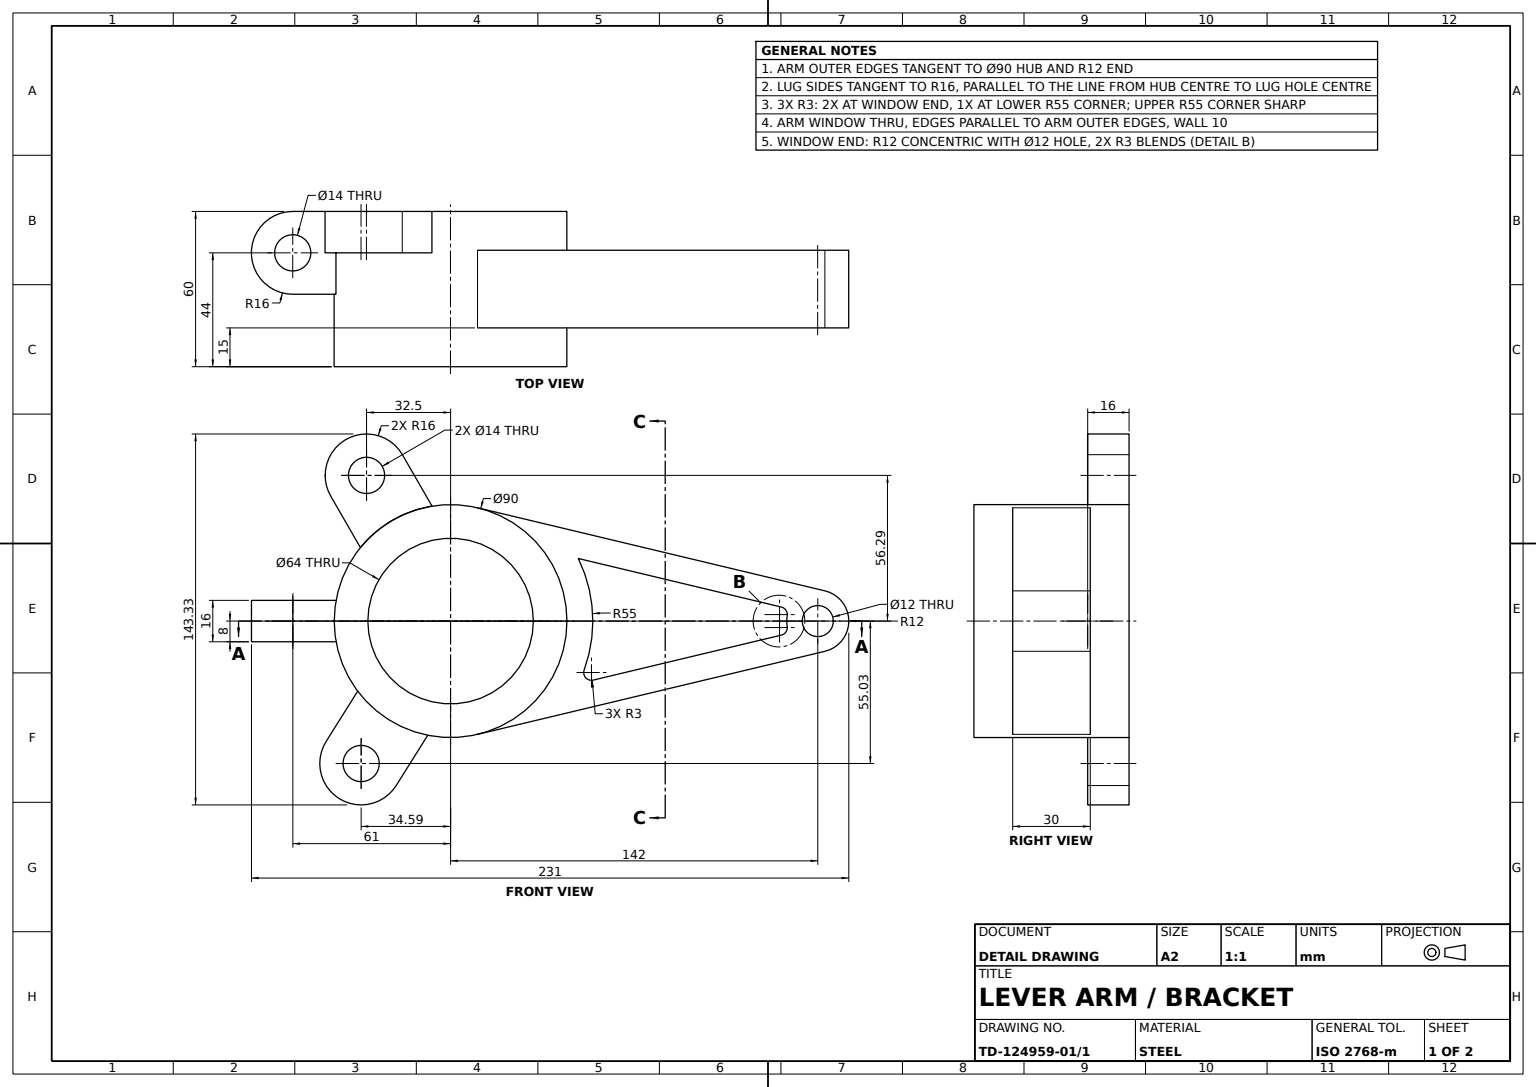
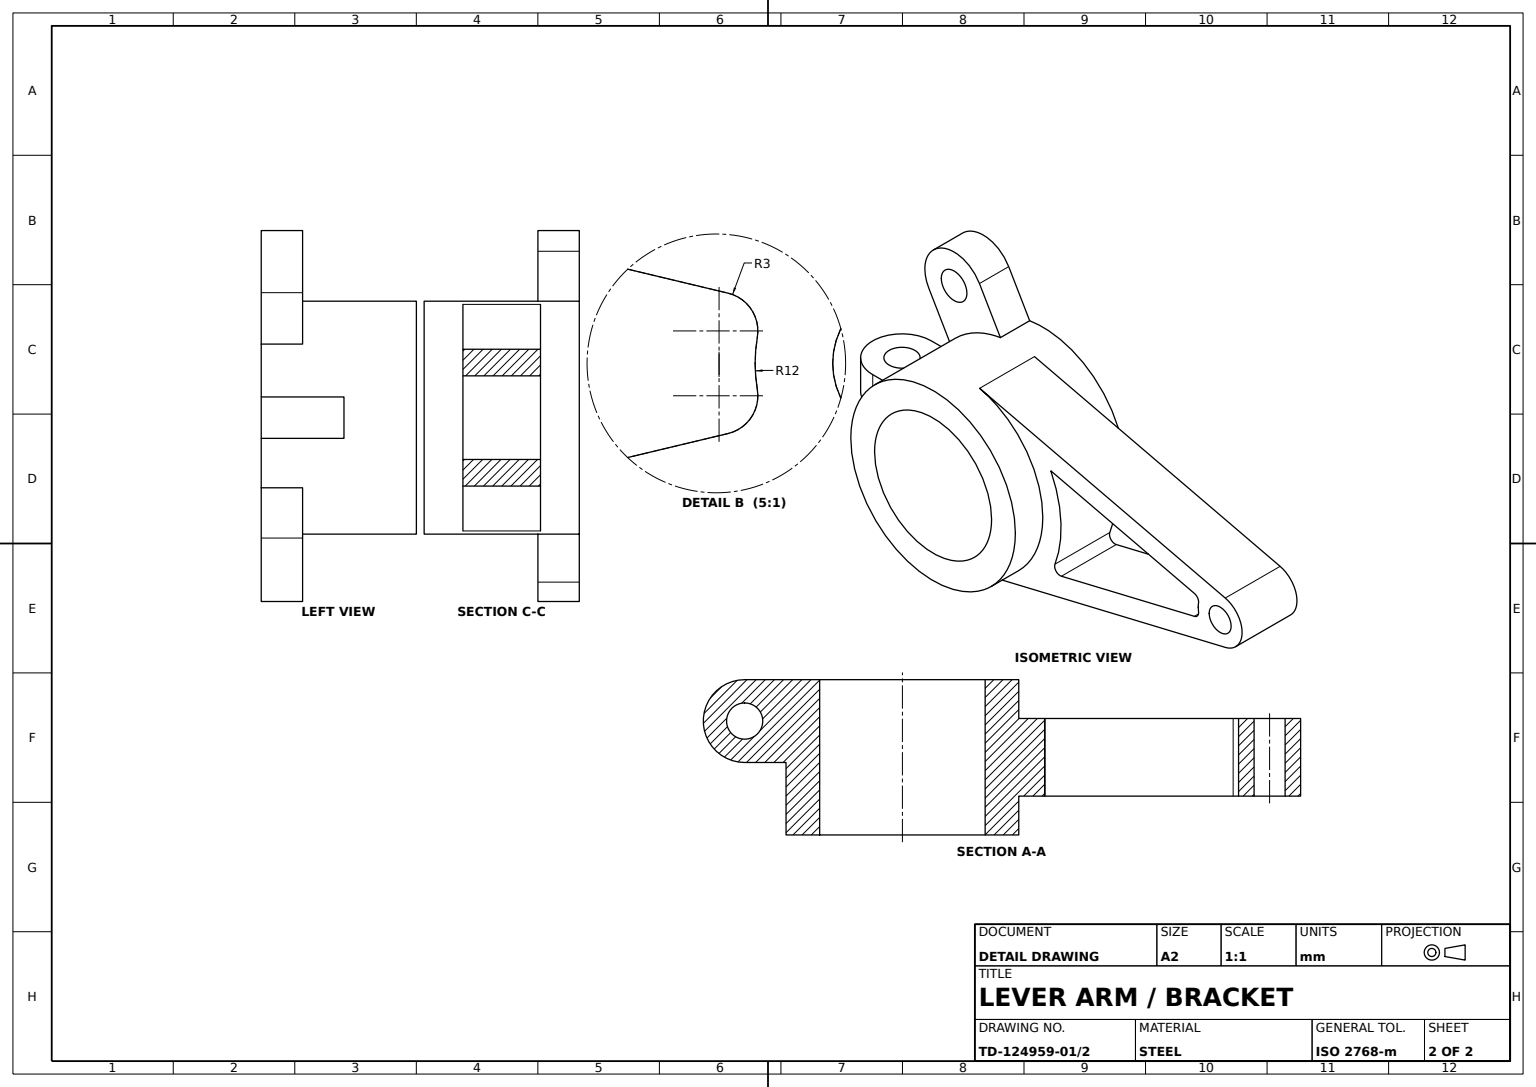
from build123d import *

# Parameters (mm, degrees)
HUB_PROFILE_90X_64_R   = 45
HUB_PROFILE_90X_64_R_2 = 32
HUB_90X_64_DEPTH       = 60
ARM_WEB_PROFILE_R      = 6
WEBBED_ARM_DEPTH       = 15
LUG_A_PROFILE_R        = 7
LUG_A_30DEG_DEPTH      = 16
LUG_B_PROFILE_R        = 7
LUG_B_30DEG_DEPTH      = 16
LUG_BOSS_DEPTH         = 8
LUG_HOLE_PROFILE_R     = 7
LUG_THROUGH_HOLE_DEPTH = 16


with BuildPart() as part:
    # Hub Profile Ø90xØ64 → Hub Ø90xØ64 (new body)
    with BuildSketch(Plane.XY):
        Circle(HUB_PROFILE_90X_64_R)
        Circle(HUB_PROFILE_90X_64_R_2, mode=Mode.SUBTRACT)
    extrude(amount=HUB_90X_64_DEPTH)

    # Arm Web Profile → Webbed Arm (add, symmetric)
    with BuildSketch(Plane.XY.offset(30)):
        with BuildLine():
            Line((10.457746479, -43.767973892), (144.788732394, -11.671459704))
            ThreePointArc((144.788732394, -11.671459704), (154, 0), (144.788732394, 11.671459704))
            Line((144.788732394, 11.671459704), (10.457746479, 43.767973892))
            ThreePointArc((10.457746479, 43.767973892), (45, 0), (10.457746479, -43.767973892))
        make_face()
        with Locations((142, 0)):
            Circle(ARM_WEB_PROFILE_R, mode=Mode.SUBTRACT)
        with BuildLine():
            ThreePointArc((127.907920927, -5.423403672), (129.71316959, -4.160179273), (130.168590262, -2.004430997))
            ThreePointArc((130.168590262, -2.004430997), (130, 0), (130.168590262, 2.004430997))
            ThreePointArc((130.168590262, 2.004430997), (129.71316959, 4.160179273), (127.907920927, 5.423403672))
            Line((127.907920927, 5.423403672), (49.398644334, 24.182099536))
            ThreePointArc((49.398644334, 24.182099536), (54.923721956, 2.89564613), (51.667548043, -18.853765651))
            ThreePointArc((51.667548043, -18.853765651), (52.245702855, -21.877663737), (55.182961035, -22.800017794))
            Line((55.182961035, -22.800017794), (127.907920927, -5.423403672))
        make_face(mode=Mode.SUBTRACT)
    extrude(amount=WEBBED_ARM_DEPTH, both=True)

    # Lug A Profile → Lug A 30deg (add)
    with BuildSketch(Plane.XY):
        with BuildLine():
            Line((-34.886147305, 28.424579613), (-46.356406461, 48.291651246))
            ThreePointArc((-46.356406461, 48.291651246), (-40.5, 70.148057707), (-18.643593539, 64.291651246))
            Line((-18.643593539, 64.291651246), (-7.173334384, 44.424579613))
            ThreePointArc((-7.173334384, 44.424579613), (-22.5, 38.97114317), (-34.886147305, 28.424579613))
        make_face()
        with Locations((-32.5, 56.291651246)):
            Circle(LUG_A_PROFILE_R, mode=Mode.SUBTRACT)
    extrude(amount=LUG_A_30DEG_DEPTH)

    # Lug B Profile → Lug B 30deg (add)
    with BuildSketch(Plane.XY):
        with BuildLine():
            ThreePointArc((-8.833624625, -44.124449866), (-23.945086023, -38.100299938), (-35.927171248, -27.096833139))
            Line((-35.927171248, -27.096833139), (-48.134119789, -46.519958213))
            ThreePointArc((-48.134119789, -46.519958213), (-43.101154841, -68.580539888), (-21.040573166, -63.547574941))
            Line((-21.040573166, -63.547574941), (-8.833624625, -44.124449866))
        make_face()
        with Locations((-34.587346477, -55.033766577)):
            Circle(LUG_B_PROFILE_R, mode=Mode.SUBTRACT)
    extrude(amount=LUG_B_30DEG_DEPTH)

    # Lug Boss Profile → Lug Boss (add, symmetric)
    with BuildSketch(Plane(origin=(0, 0, 0), x_dir=(1, 0, 0), z_dir=(0, 1, 0))):
        with BuildLine():
            Line((-61, 0), (-45, 0))
            Line((-45, 0), (-39.05307602, 0))
            Line((-39.05307602, 0), (-39.05307602, -32))
            Line((-39.05307602, -32), (-45, -32))
            Line((-45, -32), (-61, -32))
            ThreePointArc((-61, -32), (-77, -16), (-61, 0))
        make_face()
    extrude(amount=LUG_BOSS_DEPTH, both=True)

    # Lug Hole Profile → Lug Through Hole (cut)
    with BuildSketch(Plane(origin=(0, 8, 0), x_dir=(1, 0, 0), z_dir=(0, 1, 0))):
        with Locations(Location((-61, -16, 0), (0, 0, 270))):
            Circle(LUG_HOLE_PROFILE_R)
    extrude(amount=-LUG_THROUGH_HOLE_DEPTH, mode=Mode.SUBTRACT)


solid = part.part
